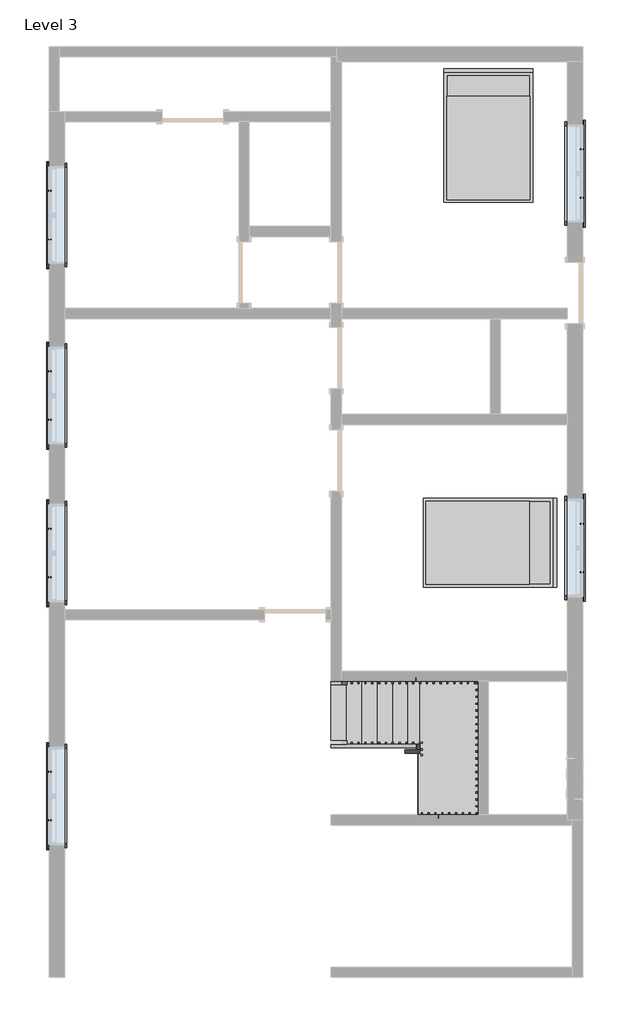
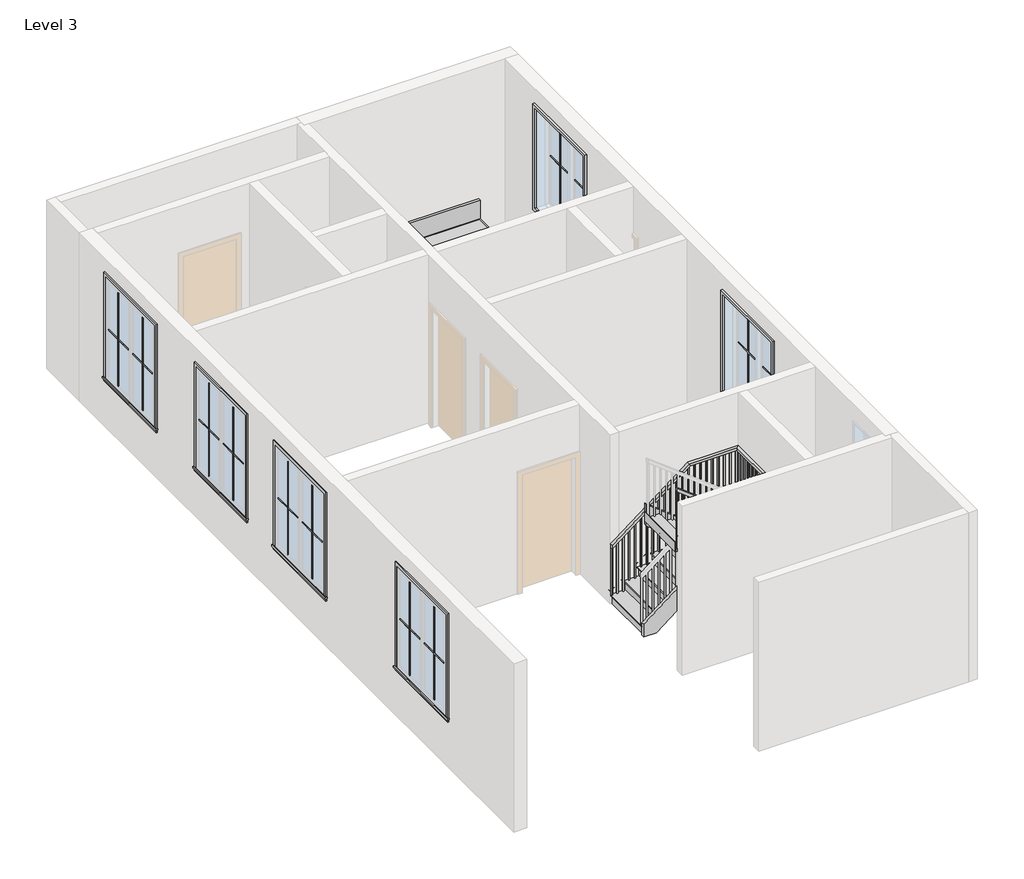
# One storey, part 2 of 2: 24 proxies, 6 members, 2 furniture elements, 1 railing, 1 stair flight.
"""IFC4 building model written with IfcOpenShell, lengths in millimetres."""

from ifc_helpers import new_model, si_unit, frame, origin, place, context, project, spatial, polyline, outline, extrude, faceted_brep, transform, mapped, element, save
from components import muntin_pattern_2x2_muntin_pattern_2x2_bff912c5, muntin_pattern_2x2_muntin_pattern_2x2_c2194282, trim_window_exterior_flat_with_sill_e04b3088, trim_window_interior_flat_picture_frame_2a7685fe, bed_17739_bed_17739_15c61121, stair_flight_9844eda0

model = new_model("IFC4")

# Units and contexts
model_context = context("Model", 3, world=origin())
ifc_project = project(units=[si_unit("LENGTHUNIT", "METRE", prefix="MILLI")], contexts=[model_context])

# Site, building, storey
site = spatial("IfcSite", under=ifc_project)
building = spatial("IfcBuilding", under=site)
storey = spatial("IfcBuildingStorey", under=building, Name="Level 3", Elevation=3200.4)

# Proxies
placement = place(None, origin())
muntin_pattern_2x2_muntin_pattern_2x2_shape = muntin_pattern_2x2_muntin_pattern_2x2_bff912c5(model_context)
element("IfcBuildingElementProxy", 1, Name="Muntin Pattern_2x2 : Muntin Pattern_2x2", ObjectType="Muntin Pattern_2x2 : Muntin Pattern_2x2", at=placement, inside=storey, context=model_context, shape_type="MappedRepresentation", body=[
    mapped(muntin_pattern_2x2_muntin_pattern_2x2_shape, transform((-5204.1165352, 3633.8812696, 4184.65), x_axis=(0.0, 1.0, 0.0), y_axis=(-1.0, 0.0, 0.0), z_axis=(0.0, 0.0, 1.0))),
])
element("IfcBuildingElementProxy", 2, Name="Muntin Pattern_2x2 : Muntin Pattern_2x2", ObjectType="Muntin Pattern_2x2 : Muntin Pattern_2x2", at=placement, inside=storey, context=model_context, shape_type="MappedRepresentation", body=[
    mapped(muntin_pattern_2x2_muntin_pattern_2x2_shape, transform((2701.6334648, 4971.3355313, 4184.65), x_axis=(0.0, -1.0, 0.0), y_axis=(1.0, 0.0, 0.0), z_axis=(0.0, 0.0, 1.0))),
])
element("IfcBuildingElementProxy", 3, Name="Muntin Pattern_2x2 : Muntin Pattern_2x2", ObjectType="Muntin Pattern_2x2 : Muntin Pattern_2x2", at=placement, inside=storey, context=model_context, shape_type="MappedRepresentation", body=[
    mapped(muntin_pattern_2x2_muntin_pattern_2x2_shape, transform((2701.6334648, -584.9144687, 4184.65), x_axis=(0.0, -1.0, 0.0), y_axis=(1.0, 0.0, 0.0), z_axis=(0.0, 0.0, 1.0))),
])
element("IfcBuildingElementProxy", 4, Name="Muntin Pattern_2x2 : Muntin Pattern_2x2", ObjectType="Muntin Pattern_2x2 : Muntin Pattern_2x2", at=placement, inside=storey, context=model_context, shape_type="MappedRepresentation", body=[
    mapped(muntin_pattern_2x2_muntin_pattern_2x2_shape, transform((-5204.1165352, 954.9605313, 4184.65), x_axis=(0.0, 1.0, 0.0), y_axis=(-1.0, 0.0, 0.0), z_axis=(0.0, 0.0, 1.0))),
])
element("IfcBuildingElementProxy", 5, Name="Muntin Pattern_2x2 : Muntin Pattern_2x2", ObjectType="Muntin Pattern_2x2 : Muntin Pattern_2x2", at=placement, inside=storey, context=model_context, shape_type="MappedRepresentation", body=[
    mapped(muntin_pattern_2x2_muntin_pattern_2x2_shape, transform((-5204.1165352, -1381.8394687, 4184.65), x_axis=(0.0, 1.0, 0.0), y_axis=(-1.0, 0.0, 0.0), z_axis=(0.0, 0.0, 1.0))),
])
element("IfcBuildingElementProxy", 6, Name="Muntin Pattern_2x2 : Muntin Pattern_2x2", ObjectType="Muntin Pattern_2x2 : Muntin Pattern_2x2", at=placement, inside=storey, context=model_context, shape_type="MappedRepresentation", body=[
    mapped(muntin_pattern_2x2_muntin_pattern_2x2_shape, transform((-5204.1165352, -4988.6394687, 4184.65), x_axis=(0.0, 1.0, 0.0), y_axis=(-1.0, 0.0, 0.0), z_axis=(0.0, 0.0, 1.0))),
])
muntin_pattern_2x2_muntin_pattern_2x2_2_shape = muntin_pattern_2x2_muntin_pattern_2x2_c2194282(model_context)
element("IfcBuildingElementProxy", 7, Name="Muntin Pattern_2x2 : Muntin Pattern_2x2", ObjectType="Muntin Pattern_2x2 : Muntin Pattern_2x2", at=placement, inside=storey, context=model_context, shape_type="MappedRepresentation", body=[
    mapped(muntin_pattern_2x2_muntin_pattern_2x2_2_shape, transform((-5204.1165352, 4354.6062696, 4184.65), x_axis=(0.0, -1.0, 0.0), y_axis=(1.0, 0.0, 0.0), z_axis=(0.0, 0.0, 1.0))),
])
element("IfcBuildingElementProxy", 8, Name="Muntin Pattern_2x2 : Muntin Pattern_2x2", ObjectType="Muntin Pattern_2x2 : Muntin Pattern_2x2", at=placement, inside=storey, context=model_context, shape_type="MappedRepresentation", body=[
    mapped(muntin_pattern_2x2_muntin_pattern_2x2_2_shape, transform((2701.6334648, 4250.6105313, 4184.65), x_axis=(0.0, 1.0, 0.0), y_axis=(-1.0, 0.0, 0.0), z_axis=(0.0, 0.0, 1.0))),
])
element("IfcBuildingElementProxy", 9, Name="Muntin Pattern_2x2 : Muntin Pattern_2x2", ObjectType="Muntin Pattern_2x2 : Muntin Pattern_2x2", at=placement, inside=storey, context=model_context, shape_type="MappedRepresentation", body=[
    mapped(muntin_pattern_2x2_muntin_pattern_2x2_2_shape, transform((2701.6334648, -1305.6394687, 4184.65), x_axis=(0.0, 1.0, 0.0), y_axis=(-1.0, 0.0, 0.0), z_axis=(0.0, 0.0, 1.0))),
])
element("IfcBuildingElementProxy", 10, Name="Muntin Pattern_2x2 : Muntin Pattern_2x2", ObjectType="Muntin Pattern_2x2 : Muntin Pattern_2x2", at=placement, inside=storey, context=model_context, shape_type="MappedRepresentation", body=[
    mapped(muntin_pattern_2x2_muntin_pattern_2x2_2_shape, transform((-5204.1165352, 1675.6855313, 4184.65), x_axis=(0.0, -1.0, 0.0), y_axis=(1.0, 0.0, 0.0), z_axis=(0.0, 0.0, 1.0))),
])
element("IfcBuildingElementProxy", 11, Name="Muntin Pattern_2x2 : Muntin Pattern_2x2", ObjectType="Muntin Pattern_2x2 : Muntin Pattern_2x2", at=placement, inside=storey, context=model_context, shape_type="MappedRepresentation", body=[
    mapped(muntin_pattern_2x2_muntin_pattern_2x2_2_shape, transform((-5204.1165352, -661.1144687, 4184.65), x_axis=(0.0, -1.0, 0.0), y_axis=(1.0, 0.0, 0.0), z_axis=(0.0, 0.0, 1.0))),
])
element("IfcBuildingElementProxy", 12, Name="Muntin Pattern_2x2 : Muntin Pattern_2x2", ObjectType="Muntin Pattern_2x2 : Muntin Pattern_2x2", at=placement, inside=storey, context=model_context, shape_type="MappedRepresentation", body=[
    mapped(muntin_pattern_2x2_muntin_pattern_2x2_2_shape, transform((-5204.1165352, -4267.9144687, 4184.65), x_axis=(0.0, -1.0, 0.0), y_axis=(1.0, 0.0, 0.0), z_axis=(0.0, 0.0, 1.0))),
])
trim_window_exterior_flat_with_sill_shape = trim_window_exterior_flat_with_sill_e04b3088(model_context)
element("IfcBuildingElementProxy", 13, Name="Trim-Window-Exterior-Flat : with Sill", ObjectType="Trim-Window-Exterior-Flat : with Sill", at=placement, inside=storey, context=model_context, shape_type="MappedRepresentation", body=[
    mapped(trim_window_exterior_flat_with_sill_shape, transform((-5213.6415352, 3994.2437696, 5943.6), x_axis=(0.0, -1.0, 0.0), y_axis=(0.0, 0.0, 1.0), z_axis=(-1.0, 0.0, 0.0))),
])
element("IfcBuildingElementProxy", 14, Name="Trim-Window-Exterior-Flat : with Sill", ObjectType="Trim-Window-Exterior-Flat : with Sill", at=placement, inside=storey, context=model_context, shape_type="MappedRepresentation", body=[
    mapped(trim_window_exterior_flat_with_sill_shape, transform((2711.1584648, 4610.9730313, 5943.6), x_axis=(0.0, 1.0, 0.0), y_axis=(0.0, 0.0, 1.0), z_axis=(1.0, 0.0, 0.0))),
])
element("IfcBuildingElementProxy", 15, Name="Trim-Window-Exterior-Flat : with Sill", ObjectType="Trim-Window-Exterior-Flat : with Sill", at=placement, inside=storey, context=model_context, shape_type="MappedRepresentation", body=[
    mapped(trim_window_exterior_flat_with_sill_shape, transform((2711.1584648, -945.2769687, 5943.6), x_axis=(0.0, 1.0, 0.0), y_axis=(0.0, 0.0, 1.0), z_axis=(1.0, 0.0, 0.0))),
])
element("IfcBuildingElementProxy", 16, Name="Trim-Window-Exterior-Flat : with Sill", ObjectType="Trim-Window-Exterior-Flat : with Sill", at=placement, inside=storey, context=model_context, shape_type="MappedRepresentation", body=[
    mapped(trim_window_exterior_flat_with_sill_shape, transform((-5213.6415352, 1315.3230313, 5943.6), x_axis=(0.0, -1.0, 0.0), y_axis=(0.0, 0.0, 1.0), z_axis=(-1.0, 0.0, 0.0))),
])
element("IfcBuildingElementProxy", 17, Name="Trim-Window-Exterior-Flat : with Sill", ObjectType="Trim-Window-Exterior-Flat : with Sill", at=placement, inside=storey, context=model_context, shape_type="MappedRepresentation", body=[
    mapped(trim_window_exterior_flat_with_sill_shape, transform((-5213.6415352, -1021.4769687, 5943.6), x_axis=(0.0, -1.0, 0.0), y_axis=(0.0, 0.0, 1.0), z_axis=(-1.0, 0.0, 0.0))),
])
element("IfcBuildingElementProxy", 18, Name="Trim-Window-Exterior-Flat : with Sill", ObjectType="Trim-Window-Exterior-Flat : with Sill", at=placement, inside=storey, context=model_context, shape_type="MappedRepresentation", body=[
    mapped(trim_window_exterior_flat_with_sill_shape, transform((-5213.6415352, -4628.2769687, 5943.6), x_axis=(0.0, -1.0, 0.0), y_axis=(0.0, 0.0, 1.0), z_axis=(-1.0, 0.0, 0.0))),
])
trim_window_interior_flat_picture_frame_shape = trim_window_interior_flat_picture_frame_2a7685fe(model_context)
element("IfcBuildingElementProxy", 19, Name="Trim-Window-Interior-Flat : Picture Frame", ObjectType="Trim-Window-Interior-Flat : Picture Frame", at=placement, inside=storey, context=model_context, shape_type="MappedRepresentation", body=[
    mapped(trim_window_interior_flat_picture_frame_shape, transform((-4985.0415352, 3994.2437696, 5943.6), x_axis=(0.0, 1.0, 0.0), y_axis=(0.0, 0.0, 1.0), z_axis=(1.0, 0.0, 0.0))),
])
element("IfcBuildingElementProxy", 20, Name="Trim-Window-Interior-Flat : Picture Frame", ObjectType="Trim-Window-Interior-Flat : Picture Frame", at=placement, inside=storey, context=model_context, shape_type="MappedRepresentation", body=[
    mapped(trim_window_interior_flat_picture_frame_shape, transform((2482.5584648, 4610.9730313, 5943.6), x_axis=(0.0, -1.0, 0.0), y_axis=(0.0, 0.0, 1.0), z_axis=(-1.0, 0.0, 0.0))),
])
element("IfcBuildingElementProxy", 21, Name="Trim-Window-Interior-Flat : Picture Frame", ObjectType="Trim-Window-Interior-Flat : Picture Frame", at=placement, inside=storey, context=model_context, shape_type="MappedRepresentation", body=[
    mapped(trim_window_interior_flat_picture_frame_shape, transform((2482.5584648, -945.2769687, 5943.6), x_axis=(0.0, -1.0, 0.0), y_axis=(0.0, 0.0, 1.0), z_axis=(-1.0, 0.0, 0.0))),
])
element("IfcBuildingElementProxy", 22, Name="Trim-Window-Interior-Flat : Picture Frame", ObjectType="Trim-Window-Interior-Flat : Picture Frame", at=placement, inside=storey, context=model_context, shape_type="MappedRepresentation", body=[
    mapped(trim_window_interior_flat_picture_frame_shape, transform((-4985.0415352, 1315.3230313, 5943.6), x_axis=(0.0, 1.0, 0.0), y_axis=(0.0, 0.0, 1.0), z_axis=(1.0, 0.0, 0.0))),
])
element("IfcBuildingElementProxy", 23, Name="Trim-Window-Interior-Flat : Picture Frame", ObjectType="Trim-Window-Interior-Flat : Picture Frame", at=placement, inside=storey, context=model_context, shape_type="MappedRepresentation", body=[
    mapped(trim_window_interior_flat_picture_frame_shape, transform((-4985.0415352, -1021.4769687, 5943.6), x_axis=(0.0, 1.0, 0.0), y_axis=(0.0, 0.0, 1.0), z_axis=(1.0, 0.0, 0.0))),
])
element("IfcBuildingElementProxy", 24, Name="Trim-Window-Interior-Flat : Picture Frame", ObjectType="Trim-Window-Interior-Flat : Picture Frame", at=placement, inside=storey, context=model_context, shape_type="MappedRepresentation", body=[
    mapped(trim_window_interior_flat_picture_frame_shape, transform((-4985.0415352, -4628.2769687, 5943.6), x_axis=(0.0, 1.0, 0.0), y_axis=(0.0, 0.0, 1.0), z_axis=(1.0, 0.0, 0.0))),
])

# Furniture
bed_17739_bed_17739_shape = bed_17739_bed_17739_15c61121(model_context)
element("IfcFurniture", 25, ObjectType="Bed_17739 : Bed_17739", at=placement, inside=storey, context=model_context, shape_type="MappedRepresentation", body=[
    mapped(bed_17739_bed_17739_shape, transform((1314.1584648, 5149.1645078, 3200.4), x_axis=(1.0, 0.0, 0.0), y_axis=(0.0, 1.0, 0.0), z_axis=(0.0, 0.0, 1.0))),
])
element("IfcFurniture", 26, ObjectType="Bed_17739 : Bed_17739", at=placement, inside=storey, context=model_context, shape_type="MappedRepresentation", body=[
    mapped(bed_17739_bed_17739_shape, transform((1314.1584648, -869.0769687, 3200.4), x_axis=(0.0, -1.0, 0.0), y_axis=(1.0, 0.0, 0.0), z_axis=(0.0, 0.0, 1.0))),
])

# Members
element("IfcMember", 27, ObjectType="Stringer - 2\" Width", at=placement, inside=storey, context=model_context, shape_type="SweptSolid", body=[
    extrude(outline(polyline([(3422.1399812, -1022.6415352), (3200.4, -1022.6415352), (3200.4, -811.2687863), (4461.9333333, 810.8400359), (4461.9333333, 314.3488758), (3422.1399812, -1022.6415352)])), frame((0.0, -2926.4769687, 0.0), z_axis=(0.0, 1.0, 0.0), x_axis=(0.0, 0.0, 1.0)), (0.0, 0.0, 1.0), 50.8),
])
element("IfcMember", 28, ObjectType="Stringer - 2\" Width", at=placement, inside=storey, context=model_context, shape_type="SweptSolid", body=[
    extrude(outline(polyline([(1161.7584648, -2875.6769687), (1212.5584648, -2875.6769687), (1212.5584648, -4907.6769687), (1161.7584648, -4907.6769687), (1161.7584648, -2875.6769687)])), frame((0.0, 0.0, 4157.1333333), z_axis=(0.0, 0.0, 1.0), x_axis=(1.0, 0.0, 0.0)), (0.0, 0.0, 1.0), 304.8),
])
element("IfcMember", 29, ObjectType="Stringer - 2\" Width", at=placement, inside=storey, context=model_context, shape_type="SweptSolid", body=[
    extrude(outline(polyline([(4157.1333333, 884.5469698), (5640.3765283, -1022.6415352), (5254.2494451, -1022.6415352), (4157.1333333, 388.0558097), (4157.1333333, 884.5469698)])), frame((0.0, -4958.4769687, 0.0), z_axis=(0.0, 1.0, 0.0), x_axis=(0.0, 0.0, 1.0)), (0.0, 0.0, 1.0), 50.8),
])
element("IfcMember", 30, ObjectType="Stringer - 2\" Width", at=placement, inside=storey, context=model_context, shape_type="SweptSolid", body=[
    extrude(outline(polyline([(3422.1399812, -1022.6415352), (3200.4, -1022.6415352), (3200.4, -811.2687863), (4020.9567404, 243.8221038), (4407.0838236, 243.8221038), (3422.1399812, -1022.6415352)])), frame((0.0, -3912.0539367, 0.0), z_axis=(0.0, 1.0, 0.0), x_axis=(0.0, 0.0, 1.0)), (0.0, 0.0, 1.0), 50.8),
])
element("IfcMember", 31, ObjectType="Stringer - 2\" Width", at=placement, inside=storey, context=model_context, shape_type="SweptSolid", body=[
    extrude(outline(polyline([(243.8221038, -3861.2539367), (294.6221038, -3861.2539367), (294.6221038, -3942.4769687), (243.8221038, -3942.4769687), (243.8221038, -3861.2539367)])), frame((0.0, 0.0, 4157.1333333), z_axis=(0.0, 0.0, 1.0), x_axis=(1.0, 0.0, 0.0)), (0.0, 0.0, 1.0), 304.8),
])
element("IfcMember", 32, ObjectType="Stringer - 2\" Width", at=placement, inside=storey, context=model_context, shape_type="SweptSolid", body=[
    extrude(outline(polyline([(4229.7978382, 294.6221038), (4615.9249214, 294.6221038), (5640.3765283, -1022.6415352), (5254.2494451, -1022.6415352), (4229.7978382, 294.6221038)])), frame((0.0, -3993.2769687, 0.0), z_axis=(0.0, 1.0, 0.0), x_axis=(0.0, 0.0, 1.0)), (0.0, 0.0, 1.0), 50.8),
])

# Railing
element("IfcRailing", 33, ObjectType="Handrail - Rectangular", at=placement, inside=storey, context=model_context, shape_type="SolidModel", body=[
    faceted_brep([(-1022.6415352, -2926.4769687, 4284.1333333), (-1022.6415352, -2926.4769687, 4219.9783974), (-1022.6415352, -2977.2769687, 4219.9783974), (-1022.6415352, -2977.2769687, 4284.1333333), (294.6221038, -2926.4769687, 5300.1333333), (311.9370364, -2926.4769687, 5249.3333333), (311.9370364, -2977.2769687, 5249.3333333), (294.6221038, -2977.2769687, 5300.1333333), (1161.7584648, -2926.4769687, 5300.1333333), (1161.7584648, -2926.4769687, 5249.3333333), (1110.9584648, -2977.2769687, 5249.3333333), (1110.9584648, -2977.2769687, 5300.1333333), (1161.7584648, -4907.6769687, 5300.1333333), (1161.7584648, -4907.6769687, 5249.3333333), (1110.9584648, -4856.8769687, 5249.3333333), (1110.9584648, -4856.8769687, 5300.1333333), (514.1660437, -4907.6769687, 5300.1333333), (496.8511111, -4907.6769687, 5249.3333333), (496.8511111, -4856.8769687, 5249.3333333), (514.1660437, -4856.8769687, 5300.1333333), (-1022.6415352, -4907.6769687, 6485.4666667), (-1022.6415352, -4856.8769687, 6485.4666667), (-1022.6415352, -4856.8769687, 6421.3117307), (-1022.6415352, -4907.6769687, 6421.3117307)], [[[0, 1, 2, 3]], [[1, 0, 4, 5]], [[2, 1, 5, 6]], [[3, 2, 6, 7]], [[0, 3, 7, 4]], [[5, 4, 8, 9]], [[6, 5, 9, 10]], [[7, 6, 10, 11]], [[4, 7, 11, 8]], [[9, 8, 12, 13]], [[10, 9, 13, 14]], [[11, 10, 14, 15]], [[8, 11, 15, 12]], [[13, 12, 16, 17]], [[14, 13, 17, 18]], [[15, 14, 18, 19]], [[12, 15, 19, 16]], [[20, 21, 22, 23]], [[17, 16, 20, 23]], [[18, 17, 23, 22]], [[19, 18, 22, 21]], [[16, 19, 21, 20]]]),
    extrude(outline(polyline([(6409.0674089, -1006.7665352), (5401.7333333, -1006.7665352), (5401.7333333, -987.7165352), (6394.3742226, -987.7165352), (6409.0674089, -1006.7665352)])), frame((0.0, -4891.8019687, 0.0), z_axis=(0.0, 1.0, 0.0), x_axis=(0.0, 0.0, 1.0)), (0.0, 0.0, 1.0), 19.05),
    extrude(outline(polyline([(6330.7037488, -905.1665352), (5401.7333333, -905.1665352), (5401.7333333, -886.1165352), (6316.0105626, -886.1165352), (6330.7037488, -905.1665352)])), frame((0.0, -4891.8019687, 0.0), z_axis=(0.0, 1.0, 0.0), x_axis=(0.0, 0.0, 1.0)), (0.0, 0.0, 1.0), 19.05),
    extrude(outline(polyline([(6252.3400888, -803.5665352), (5401.7333333, -803.5665352), (5401.7333333, -784.5165352), (6237.6469025, -784.5165352), (6252.3400888, -803.5665352)])), frame((0.0, -4891.8019687, 0.0), z_axis=(0.0, 1.0, 0.0), x_axis=(0.0, 0.0, 1.0)), (0.0, 0.0, 1.0), 19.05),
    extrude(outline(polyline([(6173.9764287, -701.9665352), (5232.4, -701.9665352), (5232.4, -682.9165352), (6159.2832425, -682.9165352), (6173.9764287, -701.9665352)])), frame((0.0, -4891.8019687, 0.0), z_axis=(0.0, 1.0, 0.0), x_axis=(0.0, 0.0, 1.0)), (0.0, 0.0, 1.0), 19.05),
    extrude(outline(polyline([(6095.6127687, -600.3665352), (5232.4, -600.3665352), (5232.4, -581.3165352), (6080.9195824, -581.3165352), (6095.6127687, -600.3665352)])), frame((0.0, -4891.8019687, 0.0), z_axis=(0.0, 1.0, 0.0), x_axis=(0.0, 0.0, 1.0)), (0.0, 0.0, 1.0), 19.05),
    extrude(outline(polyline([(6017.2491086, -498.7665352), (5063.0666667, -498.7665352), (5063.0666667, -479.7165352), (6002.5559224, -479.7165352), (6017.2491086, -498.7665352)])), frame((0.0, -4891.8019687, 0.0), z_axis=(0.0, 1.0, 0.0), x_axis=(0.0, 0.0, 1.0)), (0.0, 0.0, 1.0), 19.05),
    extrude(outline(polyline([(5938.8854486, -397.1665352), (5063.0666667, -397.1665352), (5063.0666667, -378.1165352), (5924.1922623, -378.1165352), (5938.8854486, -397.1665352)])), frame((0.0, -4891.8019687, 0.0), z_axis=(0.0, 1.0, 0.0), x_axis=(0.0, 0.0, 1.0)), (0.0, 0.0, 1.0), 19.05),
    extrude(outline(polyline([(5860.5217885, -295.5665352), (4893.7333333, -295.5665352), (4893.7333333, -276.5165352), (5845.8286023, -276.5165352), (5860.5217885, -295.5665352)])), frame((0.0, -4891.8019687, 0.0), z_axis=(0.0, 1.0, 0.0), x_axis=(0.0, 0.0, 1.0)), (0.0, 0.0, 1.0), 19.05),
    extrude(outline(polyline([(5782.1581285, -193.9665352), (4893.7333333, -193.9665352), (4893.7333333, -174.9165352), (5767.4649422, -174.9165352), (5782.1581285, -193.9665352)])), frame((0.0, -4891.8019687, 0.0), z_axis=(0.0, 1.0, 0.0), x_axis=(0.0, 0.0, 1.0)), (0.0, 0.0, 1.0), 19.05),
    extrude(outline(polyline([(5703.7944684, -92.3665352), (4724.4, -92.3665352), (4724.4, -73.3165352), (5689.1012822, -73.3165352), (5703.7944684, -92.3665352)])), frame((0.0, -4891.8019687, 0.0), z_axis=(0.0, 1.0, 0.0), x_axis=(0.0, 0.0, 1.0)), (0.0, 0.0, 1.0), 19.05),
    extrude(outline(polyline([(5625.4308084, 9.2334648), (4724.4, 9.2334648), (4724.4, 28.2834648), (5610.7376221, 28.2834648), (5625.4308084, 9.2334648)])), frame((0.0, -4891.8019687, 0.0), z_axis=(0.0, 1.0, 0.0), x_axis=(0.0, 0.0, 1.0)), (0.0, 0.0, 1.0), 19.05),
    extrude(outline(polyline([(5547.0671484, 110.8334648), (4724.4, 110.8334648), (4724.4, 129.8834648), (5532.3739621, 129.8834648), (5547.0671484, 110.8334648)])), frame((0.0, -4891.8019687, 0.0), z_axis=(0.0, 1.0, 0.0), x_axis=(0.0, 0.0, 1.0)), (0.0, 0.0, 1.0), 19.05),
    extrude(outline(polyline([(5468.7034883, 212.4334648), (4555.0666667, 212.4334648), (4555.0666667, 231.4834648), (5454.0103021, 231.4834648), (5468.7034883, 212.4334648)])), frame((0.0, -4891.8019687, 0.0), z_axis=(0.0, 1.0, 0.0), x_axis=(0.0, 0.0, 1.0)), (0.0, 0.0, 1.0), 19.05),
    extrude(outline(polyline([(5390.3398283, 314.0334648), (4385.7333333, 314.0334648), (4385.7333333, 333.0834648), (5375.646642, 333.0834648), (5390.3398283, 314.0334648)])), frame((0.0, -4891.8019687, 0.0), z_axis=(0.0, 1.0, 0.0), x_axis=(0.0, 0.0, 1.0)), (0.0, 0.0, 1.0), 19.05),
    extrude(outline(polyline([(5311.9761682, 415.6334648), (4385.7333333, 415.6334648), (4385.7333333, 434.6834648), (5297.282982, 434.6834648), (5311.9761682, 415.6334648)])), frame((0.0, -4891.8019687, 0.0), z_axis=(0.0, 1.0, 0.0), x_axis=(0.0, 0.0, 1.0)), (0.0, 0.0, 1.0), 19.05),
    extrude(outline(polyline([(536.2834648, -4891.8019687), (517.2334648, -4891.8019687), (517.2334648, -4872.7519687), (536.2834648, -4872.7519687), (536.2834648, -4891.8019687)])), frame((0.0, 0.0, 4385.7333333), z_axis=(0.0, 0.0, 1.0), x_axis=(1.0, 0.0, 0.0)), (0.0, 0.0, 1.0), 863.6),
    extrude(outline(polyline([(637.8834648, -4891.8019687), (618.8334648, -4891.8019687), (618.8334648, -4872.7519687), (637.8834648, -4872.7519687), (637.8834648, -4891.8019687)])), frame((0.0, 0.0, 4385.7333333), z_axis=(0.0, 0.0, 1.0), x_axis=(1.0, 0.0, 0.0)), (0.0, 0.0, 1.0), 863.6),
    extrude(outline(polyline([(739.4834648, -4891.8019687), (720.4334648, -4891.8019687), (720.4334648, -4872.7519687), (739.4834648, -4872.7519687), (739.4834648, -4891.8019687)])), frame((0.0, 0.0, 4385.7333333), z_axis=(0.0, 0.0, 1.0), x_axis=(1.0, 0.0, 0.0)), (0.0, 0.0, 1.0), 863.6),
    extrude(outline(polyline([(841.0834648, -4891.8019687), (822.0334648, -4891.8019687), (822.0334648, -4872.7519687), (841.0834648, -4872.7519687), (841.0834648, -4891.8019687)])), frame((0.0, 0.0, 4385.7333333), z_axis=(0.0, 0.0, 1.0), x_axis=(1.0, 0.0, 0.0)), (0.0, 0.0, 1.0), 863.6),
    extrude(outline(polyline([(942.6834648, -4891.8019687), (923.6334648, -4891.8019687), (923.6334648, -4872.7519687), (942.6834648, -4872.7519687), (942.6834648, -4891.8019687)])), frame((0.0, 0.0, 4385.7333333), z_axis=(0.0, 0.0, 1.0), x_axis=(1.0, 0.0, 0.0)), (0.0, 0.0, 1.0), 863.6),
    extrude(outline(polyline([(1044.2834648, -4891.8019687), (1025.2334648, -4891.8019687), (1025.2334648, -4872.7519687), (1044.2834648, -4872.7519687), (1044.2834648, -4891.8019687)])), frame((0.0, 0.0, 4385.7333333), z_axis=(0.0, 0.0, 1.0), x_axis=(1.0, 0.0, 0.0)), (0.0, 0.0, 1.0), 863.6),
    extrude(outline(polyline([(1145.8834648, -4771.1519687), (1145.8834648, -4790.2019687), (1126.8334648, -4790.2019687), (1126.8334648, -4771.1519687), (1145.8834648, -4771.1519687)])), frame((0.0, 0.0, 4385.7333333), z_axis=(0.0, 0.0, 1.0), x_axis=(1.0, 0.0, 0.0)), (0.0, 0.0, 1.0), 863.6),
    extrude(outline(polyline([(1145.8834648, -4669.5519687), (1145.8834648, -4688.6019687), (1126.8334648, -4688.6019687), (1126.8334648, -4669.5519687), (1145.8834648, -4669.5519687)])), frame((0.0, 0.0, 4385.7333333), z_axis=(0.0, 0.0, 1.0), x_axis=(1.0, 0.0, 0.0)), (0.0, 0.0, 1.0), 863.6),
    extrude(outline(polyline([(1145.8834648, -4567.9519687), (1145.8834648, -4587.0019687), (1126.8334648, -4587.0019687), (1126.8334648, -4567.9519687), (1145.8834648, -4567.9519687)])), frame((0.0, 0.0, 4385.7333333), z_axis=(0.0, 0.0, 1.0), x_axis=(1.0, 0.0, 0.0)), (0.0, 0.0, 1.0), 863.6),
    extrude(outline(polyline([(1145.8834648, -4466.3519687), (1145.8834648, -4485.4019687), (1126.8334648, -4485.4019687), (1126.8334648, -4466.3519687), (1145.8834648, -4466.3519687)])), frame((0.0, 0.0, 4385.7333333), z_axis=(0.0, 0.0, 1.0), x_axis=(1.0, 0.0, 0.0)), (0.0, 0.0, 1.0), 863.6),
    extrude(outline(polyline([(1145.8834648, -4364.7519687), (1145.8834648, -4383.8019687), (1126.8334648, -4383.8019687), (1126.8334648, -4364.7519687), (1145.8834648, -4364.7519687)])), frame((0.0, 0.0, 4385.7333333), z_axis=(0.0, 0.0, 1.0), x_axis=(1.0, 0.0, 0.0)), (0.0, 0.0, 1.0), 863.6),
    extrude(outline(polyline([(1145.8834648, -4263.1519687), (1145.8834648, -4282.2019687), (1126.8334648, -4282.2019687), (1126.8334648, -4263.1519687), (1145.8834648, -4263.1519687)])), frame((0.0, 0.0, 4385.7333333), z_axis=(0.0, 0.0, 1.0), x_axis=(1.0, 0.0, 0.0)), (0.0, 0.0, 1.0), 863.6),
    extrude(outline(polyline([(1145.8834648, -4161.5519687), (1145.8834648, -4180.6019687), (1126.8334648, -4180.6019687), (1126.8334648, -4161.5519687), (1145.8834648, -4161.5519687)])), frame((0.0, 0.0, 4385.7333333), z_axis=(0.0, 0.0, 1.0), x_axis=(1.0, 0.0, 0.0)), (0.0, 0.0, 1.0), 863.6),
    extrude(outline(polyline([(1145.8834648, -4059.9519687), (1145.8834648, -4079.0019687), (1126.8334648, -4079.0019687), (1126.8334648, -4059.9519687), (1145.8834648, -4059.9519687)])), frame((0.0, 0.0, 4385.7333333), z_axis=(0.0, 0.0, 1.0), x_axis=(1.0, 0.0, 0.0)), (0.0, 0.0, 1.0), 863.6),
    extrude(outline(polyline([(1145.8834648, -3958.3519687), (1145.8834648, -3977.4019687), (1126.8334648, -3977.4019687), (1126.8334648, -3958.3519687), (1145.8834648, -3958.3519687)])), frame((0.0, 0.0, 4385.7333333), z_axis=(0.0, 0.0, 1.0), x_axis=(1.0, 0.0, 0.0)), (0.0, 0.0, 1.0), 863.6),
    extrude(outline(polyline([(1145.8834648, -3856.7519687), (1145.8834648, -3875.8019687), (1126.8334648, -3875.8019687), (1126.8334648, -3856.7519687), (1145.8834648, -3856.7519687)])), frame((0.0, 0.0, 4385.7333333), z_axis=(0.0, 0.0, 1.0), x_axis=(1.0, 0.0, 0.0)), (0.0, 0.0, 1.0), 863.6),
    extrude(outline(polyline([(1145.8834648, -3755.1519687), (1145.8834648, -3774.2019687), (1126.8334648, -3774.2019687), (1126.8334648, -3755.1519687), (1145.8834648, -3755.1519687)])), frame((0.0, 0.0, 4385.7333333), z_axis=(0.0, 0.0, 1.0), x_axis=(1.0, 0.0, 0.0)), (0.0, 0.0, 1.0), 863.6),
    extrude(outline(polyline([(1145.8834648, -3653.5519687), (1145.8834648, -3672.6019687), (1126.8334648, -3672.6019687), (1126.8334648, -3653.5519687), (1145.8834648, -3653.5519687)])), frame((0.0, 0.0, 4385.7333333), z_axis=(0.0, 0.0, 1.0), x_axis=(1.0, 0.0, 0.0)), (0.0, 0.0, 1.0), 863.6),
    extrude(outline(polyline([(1145.8834648, -3551.9519687), (1145.8834648, -3571.0019687), (1126.8334648, -3571.0019687), (1126.8334648, -3551.9519687), (1145.8834648, -3551.9519687)])), frame((0.0, 0.0, 4385.7333333), z_axis=(0.0, 0.0, 1.0), x_axis=(1.0, 0.0, 0.0)), (0.0, 0.0, 1.0), 863.6),
    extrude(outline(polyline([(1145.8834648, -3450.3519687), (1145.8834648, -3469.4019687), (1126.8334648, -3469.4019687), (1126.8334648, -3450.3519687), (1145.8834648, -3450.3519687)])), frame((0.0, 0.0, 4385.7333333), z_axis=(0.0, 0.0, 1.0), x_axis=(1.0, 0.0, 0.0)), (0.0, 0.0, 1.0), 863.6),
    extrude(outline(polyline([(1145.8834648, -3348.7519687), (1145.8834648, -3367.8019687), (1126.8334648, -3367.8019687), (1126.8334648, -3348.7519687), (1145.8834648, -3348.7519687)])), frame((0.0, 0.0, 4385.7333333), z_axis=(0.0, 0.0, 1.0), x_axis=(1.0, 0.0, 0.0)), (0.0, 0.0, 1.0), 863.6),
    extrude(outline(polyline([(1145.8834648, -3247.1519687), (1145.8834648, -3266.2019687), (1126.8334648, -3266.2019687), (1126.8334648, -3247.1519687), (1145.8834648, -3247.1519687)])), frame((0.0, 0.0, 4385.7333333), z_axis=(0.0, 0.0, 1.0), x_axis=(1.0, 0.0, 0.0)), (0.0, 0.0, 1.0), 863.6),
    extrude(outline(polyline([(1145.8834648, -3145.5519687), (1145.8834648, -3164.6019687), (1126.8334648, -3164.6019687), (1126.8334648, -3145.5519687), (1145.8834648, -3145.5519687)])), frame((0.0, 0.0, 4385.7333333), z_axis=(0.0, 0.0, 1.0), x_axis=(1.0, 0.0, 0.0)), (0.0, 0.0, 1.0), 863.6),
    extrude(outline(polyline([(1145.8834648, -3043.9519687), (1145.8834648, -3063.0019687), (1126.8334648, -3063.0019687), (1126.8334648, -3043.9519687), (1145.8834648, -3043.9519687)])), frame((0.0, 0.0, 4385.7333333), z_axis=(0.0, 0.0, 1.0), x_axis=(1.0, 0.0, 0.0)), (0.0, 0.0, 1.0), 863.6),
    extrude(outline(polyline([(1101.4334648, -2942.3519687), (1120.4834648, -2942.3519687), (1120.4834648, -2961.4019687), (1101.4334648, -2961.4019687), (1101.4334648, -2942.3519687)])), frame((0.0, 0.0, 4385.7333333), z_axis=(0.0, 0.0, 1.0), x_axis=(1.0, 0.0, 0.0)), (0.0, 0.0, 1.0), 863.6),
    extrude(outline(polyline([(999.8334648, -2942.3519687), (1018.8834648, -2942.3519687), (1018.8834648, -2961.4019687), (999.8334648, -2961.4019687), (999.8334648, -2942.3519687)])), frame((0.0, 0.0, 4385.7333333), z_axis=(0.0, 0.0, 1.0), x_axis=(1.0, 0.0, 0.0)), (0.0, 0.0, 1.0), 863.6),
    extrude(outline(polyline([(898.2334648, -2942.3519687), (917.2834648, -2942.3519687), (917.2834648, -2961.4019687), (898.2334648, -2961.4019687), (898.2334648, -2942.3519687)])), frame((0.0, 0.0, 4385.7333333), z_axis=(0.0, 0.0, 1.0), x_axis=(1.0, 0.0, 0.0)), (0.0, 0.0, 1.0), 863.6),
    extrude(outline(polyline([(796.6334648, -2942.3519687), (815.6834648, -2942.3519687), (815.6834648, -2961.4019687), (796.6334648, -2961.4019687), (796.6334648, -2942.3519687)])), frame((0.0, 0.0, 4385.7333333), z_axis=(0.0, 0.0, 1.0), x_axis=(1.0, 0.0, 0.0)), (0.0, 0.0, 1.0), 863.6),
    extrude(outline(polyline([(695.0334648, -2942.3519687), (714.0834648, -2942.3519687), (714.0834648, -2961.4019687), (695.0334648, -2961.4019687), (695.0334648, -2942.3519687)])), frame((0.0, 0.0, 4385.7333333), z_axis=(0.0, 0.0, 1.0), x_axis=(1.0, 0.0, 0.0)), (0.0, 0.0, 1.0), 863.6),
    extrude(outline(polyline([(593.4334648, -2942.3519687), (612.4834648, -2942.3519687), (612.4834648, -2961.4019687), (593.4334648, -2961.4019687), (593.4334648, -2942.3519687)])), frame((0.0, 0.0, 4385.7333333), z_axis=(0.0, 0.0, 1.0), x_axis=(1.0, 0.0, 0.0)), (0.0, 0.0, 1.0), 863.6),
    extrude(outline(polyline([(491.8334648, -2942.3519687), (510.8834648, -2942.3519687), (510.8834648, -2961.4019687), (491.8334648, -2961.4019687), (491.8334648, -2942.3519687)])), frame((0.0, 0.0, 4385.7333333), z_axis=(0.0, 0.0, 1.0), x_axis=(1.0, 0.0, 0.0)), (0.0, 0.0, 1.0), 863.6),
    extrude(outline(polyline([(390.2334648, -2942.3519687), (409.2834648, -2942.3519687), (409.2834648, -2961.4019687), (390.2334648, -2961.4019687), (390.2334648, -2942.3519687)])), frame((0.0, 0.0, 4385.7333333), z_axis=(0.0, 0.0, 1.0), x_axis=(1.0, 0.0, 0.0)), (0.0, 0.0, 1.0), 863.6),
    extrude(outline(polyline([(288.6334648, -2942.3519687), (307.6834648, -2942.3519687), (307.6834648, -2961.4019687), (288.6334648, -2961.4019687), (288.6334648, -2942.3519687)])), frame((0.0, 0.0, 4385.7333333), z_axis=(0.0, 0.0, 1.0), x_axis=(1.0, 0.0, 0.0)), (0.0, 0.0, 1.0), 863.6),
    extrude(outline(polyline([(5152.9957248, 187.0334648), (4216.4, 187.0334648), (4216.4, 206.0834648), (5167.6889111, 206.0834648), (5152.9957248, 187.0334648)])), frame((0.0, -2961.4019687, 0.0), z_axis=(0.0, 1.0, 0.0), x_axis=(0.0, 0.0, 1.0)), (0.0, 0.0, 1.0), 19.05),
    extrude(outline(polyline([(5074.6320648, 85.4334648), (4047.0666667, 85.4334648), (4047.0666667, 104.4834648), (5089.325251, 104.4834648), (5074.6320648, 85.4334648)])), frame((0.0, -2961.4019687, 0.0), z_axis=(0.0, 1.0, 0.0), x_axis=(0.0, 0.0, 1.0)), (0.0, 0.0, 1.0), 19.05),
    extrude(outline(polyline([(4996.2684047, -16.1665352), (4047.0666667, -16.1665352), (4047.0666667, 2.8834648), (5010.961591, 2.8834648), (4996.2684047, -16.1665352)])), frame((0.0, -2961.4019687, 0.0), z_axis=(0.0, 1.0, 0.0), x_axis=(0.0, 0.0, 1.0)), (0.0, 0.0, 1.0), 19.05),
    extrude(outline(polyline([(4917.9047447, -117.7665352), (4047.0666667, -117.7665352), (4047.0666667, -98.7165352), (4932.5979309, -98.7165352), (4917.9047447, -117.7665352)])), frame((0.0, -2961.4019687, 0.0), z_axis=(0.0, 1.0, 0.0), x_axis=(0.0, 0.0, 1.0)), (0.0, 0.0, 1.0), 19.05),
    extrude(outline(polyline([(4839.5410846, -219.3665352), (3877.7333333, -219.3665352), (3877.7333333, -200.3165352), (4854.2342709, -200.3165352), (4839.5410846, -219.3665352)])), frame((0.0, -2961.4019687, 0.0), z_axis=(0.0, 1.0, 0.0), x_axis=(0.0, 0.0, 1.0)), (0.0, 0.0, 1.0), 19.05),
    extrude(outline(polyline([(4761.1774246, -320.9665352), (3877.7333333, -320.9665352), (3877.7333333, -301.9165352), (4775.8706109, -301.9165352), (4761.1774246, -320.9665352)])), frame((0.0, -2961.4019687, 0.0), z_axis=(0.0, 1.0, 0.0), x_axis=(0.0, 0.0, 1.0)), (0.0, 0.0, 1.0), 19.05),
    extrude(outline(polyline([(4682.8137645, -422.5665352), (3708.4, -422.5665352), (3708.4, -403.5165352), (4697.5069508, -403.5165352), (4682.8137645, -422.5665352)])), frame((0.0, -2961.4019687, 0.0), z_axis=(0.0, 1.0, 0.0), x_axis=(0.0, 0.0, 1.0)), (0.0, 0.0, 1.0), 19.05),
    extrude(outline(polyline([(4604.4501045, -524.1665352), (3708.4, -524.1665352), (3708.4, -505.1165352), (4619.1432908, -505.1165352), (4604.4501045, -524.1665352)])), frame((0.0, -2961.4019687, 0.0), z_axis=(0.0, 1.0, 0.0), x_axis=(0.0, 0.0, 1.0)), (0.0, 0.0, 1.0), 19.05),
    extrude(outline(polyline([(4526.0864445, -625.7665352), (3539.0666667, -625.7665352), (3539.0666667, -606.7165352), (4540.7796307, -606.7165352), (4526.0864445, -625.7665352)])), frame((0.0, -2961.4019687, 0.0), z_axis=(0.0, 1.0, 0.0), x_axis=(0.0, 0.0, 1.0)), (0.0, 0.0, 1.0), 19.05),
    extrude(outline(polyline([(4447.7227844, -727.3665352), (3539.0666667, -727.3665352), (3539.0666667, -708.3165352), (4462.4159707, -708.3165352), (4447.7227844, -727.3665352)])), frame((0.0, -2961.4019687, 0.0), z_axis=(0.0, 1.0, 0.0), x_axis=(0.0, 0.0, 1.0)), (0.0, 0.0, 1.0), 19.05),
    extrude(outline(polyline([(4369.3591244, -828.9665352), (3369.7333333, -828.9665352), (3369.7333333, -809.9165352), (4384.0523106, -809.9165352), (4369.3591244, -828.9665352)])), frame((0.0, -2961.4019687, 0.0), z_axis=(0.0, 1.0, 0.0), x_axis=(0.0, 0.0, 1.0)), (0.0, 0.0, 1.0), 19.05),
    extrude(outline(polyline([(4290.9954643, -930.5665352), (3369.7333333, -930.5665352), (3369.7333333, -911.5165352), (4305.6886506, -911.5165352), (4290.9954643, -930.5665352)])), frame((0.0, -2961.4019687, 0.0), z_axis=(0.0, 1.0, 0.0), x_axis=(0.0, 0.0, 1.0)), (0.0, 0.0, 1.0), 19.05),
    extrude(outline(polyline([(1145.8834648, -4872.7519687), (1145.8834648, -4891.8019687), (1126.8334648, -4891.8019687), (1126.8334648, -4872.7519687), (1145.8834648, -4872.7519687)])), frame((0.0, 0.0, 4385.7333333), z_axis=(0.0, 0.0, 1.0), x_axis=(1.0, 0.0, 0.0)), (0.0, 0.0, 1.0), 863.6),
    extrude(outline(polyline([(1126.8334648, -2942.3519687), (1145.8834648, -2942.3519687), (1145.8834648, -2961.4019687), (1126.8334648, -2961.4019687), (1126.8334648, -2942.3519687)])), frame((0.0, 0.0, 4385.7333333), z_axis=(0.0, 0.0, 1.0), x_axis=(1.0, 0.0, 0.0)), (0.0, 0.0, 1.0), 863.6),
    extrude(outline(polyline([(6421.3117307, -1022.6415352), (5401.7333333, -1022.6415352), (5401.7333333, -1003.5915352), (6406.6185445, -1003.5915352), (6421.3117307, -1022.6415352)])), frame((0.0, -4891.8019687, 0.0), z_axis=(0.0, 1.0, 0.0), x_axis=(0.0, 0.0, 1.0)), (0.0, 0.0, 1.0), 19.05),
    extrude(outline(polyline([(4219.9783974, -1022.6415352), (3369.7333333, -1022.6415352), (3369.7333333, -1003.5915352), (4234.6715837, -1003.5915352), (4219.9783974, -1022.6415352)])), frame((0.0, -2961.4019687, 0.0), z_axis=(0.0, 1.0, 0.0), x_axis=(0.0, 0.0, 1.0)), (0.0, 0.0, 1.0), 19.05),
])

# Stair flight
stair_flight_shape = stair_flight_9844eda0(model_context)
element("IfcStairFlight", 34, ObjectType="2\" Tread 1\" Nosing 1/4\" Riser", at=placement, inside=storey, context=model_context, shape_type="MappedRepresentation", body=[
    mapped(stair_flight_shape, transform((0.0, 0.0, 0.0), x_axis=(1.0, 0.0, 0.0), y_axis=(0.0, 1.0, 0.0), z_axis=(0.0, 0.0, 1.0))),
])

save(model, "model.ifc")

# Revit data of these elements
# Type "Muntin Pattern_2x2 : Muntin Pattern_2x2"
#   Width [instance default] = 4' - 0"
#   Thickness = 0' - 0 1/2"
#   Height [instance default] = 4' - 0"
#   Distance = 0' - 0 3/4"
#   Interior Material [instance default] = none
#   Exterior Material [instance default] = none
#   Default Elevation = 0
# Type "Trim-Window-Exterior-Flat : with Sill"
#   Trim Width = 0' - 2 1/4"
#   Trim Thickness_Picture Frame = 0' - 1 1/4"
#   Trim Thickness_with Sill = 0' - 0 3/4"
#   Sill Thickness = 0' - 1 1/4"
#   Opening Width [instance default] = 2' - 0"
#   Opening Height [instance default] = 3' - 0"
#   Default Elevation = 4' - 0"
#   Sill = yes
#   Picture Frame = no
#   Trim Material [instance default] = none
# Type "Trim-Window-Interior-Flat : Picture Frame"
#   Trim Thickness_Picture Frame = 0' - 1 1/4"
#   Trim Width = 0' - 2 1/4"
#   Trim Thickness_with Sill = 0' - 0 3/4"
#   Sill Thickness = 0' - 1 1/4"
#   Opening Width [instance default] = 2' - 0"
#   Opening Height [instance default] = 3' - 0"
#   Default Elevation = 4' - 0"
#   Sill = no
#   Picture Frame = yes
#   Trim Material [instance default] = none
# Type "Bed_17739 : Bed_17739"
#   Default Elevation = 0
# Type "Handrail - Rectangular"
#   Assembly Code = "C2010400"
#   built-in parameter 1008612 = 0.0416667 (stored number, unit not read)
#   built-in parameter 1008611 = 0.0416667 (stored number, unit not read)
#   built-in parameter 1008609 = 0.333333 (stored number, unit not read)
#   built-in parameter 1008604 = 0.166667 (stored number, unit not read)
#   built-in parameter 1008603 = 0.166667 (stored number, unit not read)
#   Railing Height = 3' - 0"
#   built-in parameter 1008630 = 2
#   built-in parameter 1008610 = 2
#   built-in parameter 1008618 = Baluster - Square : 3/4"
# Elements 1, 2, 3, 4, 5, 6, 7, 8, 9, 10, 11, 12 (IfcBuildingElementProxy, "Muntin Pattern_2x2 : Muntin Pattern_2x2")
#   Width = 1' - 11 1/8"
#   Height = 5' - 6 1/2"
#   Interior Material = Wood - Stained
#   Exterior Material = Clad - White
#   Phase Created = New Construction
#   Materials on its faces: "Clad - White", "Wood - Stained"
# Elements 13, 14, 15, 16, 17, 18 (IfcBuildingElementProxy, "Trim-Window-Exterior-Flat : with Sill")
#   Opening Width = 4' - 9"
#   Opening Height = 6' - 0"
#   Trim Material = Clad - White
#   Phase Created = New Construction
#   Materials on its faces: "Clad - White"
# Elements 19, 20, 21, 22, 23, 24 (IfcBuildingElementProxy, "Trim-Window-Interior-Flat : Picture Frame")
#   Opening Width = 4' - 9"
#   Opening Height = 6' - 0"
#   Trim Material = Wood - Stained
#   Phase Created = New Construction
#   Materials on its faces: "Wood - Stained"
# Elements 25, 26 (IfcFurniture, "Bed_17739 : Bed_17739")
#   Phase Created = New Construction
#   Materials on its faces: "legs", "sheets", "bed frame", "Blanket"
# Elements 27, 28, 29, 30, 31, 32 (IfcMember, "Stringer - 2\" Width")
#   Phase Created = New Construction
# Element 33 (IfcRailing, "Handrail - Rectangular")
#   Phase Created = New Construction
# Element 34 (IfcStairFlight, "2\" Tread 1\" Nosing 1/4\" Riser")
#   Phase Created = New Construction
# Materials
#   "Clad - White": class "Wood", colour RGB 242 242 238, transparency 0, Cost = 0
#   "Wood - Stained": class "Wood", colour RGB 224 178 126, transparency 0, Cost = 0
#   "legs": colour RGB 90 73 37, transparency 0, Cost = 0
#   "sheets": colour RGB 200 195 176, transparency 0, Cost = 0
#   "bed frame": colour RGB 90 73 37, transparency 0, Cost = 0
#   "Blanket": class "System", colour RGB 59 0 1, transparency 0, Cost = 0
